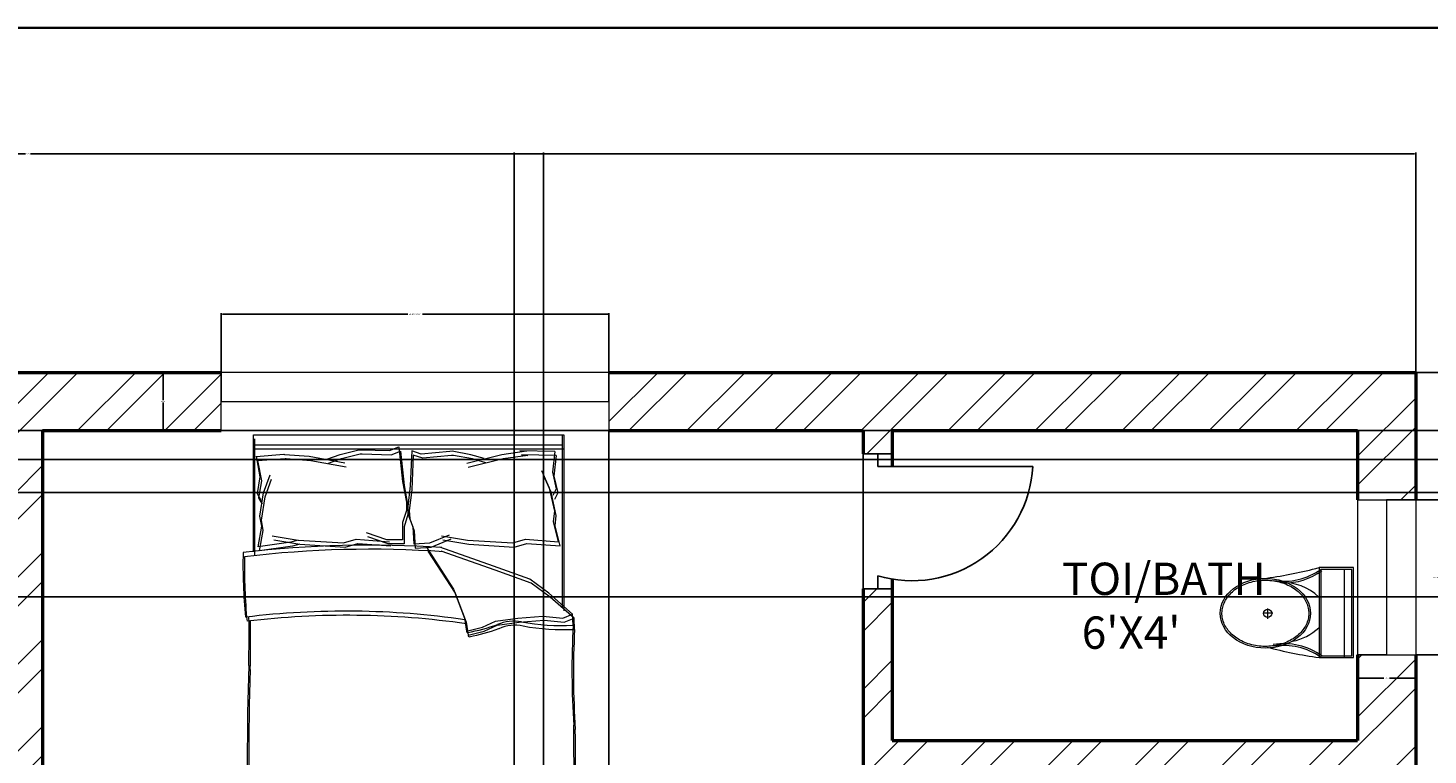
# Model space of a CAD drawing. Units: inches. Extents: x 2310 to 2937, y 1113 to 2410.
# Tile 22 of 23: x 2609 to 2826, y 2297 to 2410. Entities that reach past the tile are written whole.
import ezdxf

# ---------------------------------------------------------------- set-up
doc = ezdxf.new("R2010")
doc.units = ezdxf.units.IN
for name, color, linetype, lineweight in [('A-ANNO-DIMS', 2, 'Continuous', 18), ('A-ANNO-TTLB', 7, 'Continuous', 35), ('A-AREA-IDEN', 7, 'Continuous', 18), ('A-DOOR', 31, 'Continuous', 25), ('A-FLOR-FIXT', 9, 'Continuous', 18), ('A-FURN', 8, 'Continuous', 18), ('A-GLAZ', 191, 'Continuous', 20), ('A-WALL', 7, 'Continuous', 50), ('A-WALL-PATT', 85, 'Continuous', 13)]:
    doc.layers.add(name, color=color, linetype=linetype, lineweight=lineweight)
doc.styles.get("Standard").update_dxf_attribs({"font": 'arial.ttf'})
doc.dimstyles.get("Standard").update_dxf_attribs({"dimtxt": 0.18, "dimasz": 0.18, "dimexe": 0.18, "dimexo": 0.0625, "dimgap": 0.09, "dimtad": 0, "dimtih": 1, "dimtoh": 1, "dimdec": 4, "dimzin": 0, "dimdsep": 46, "dimtxsty": 'Standard', "dimcen": 0.09, "dimadec": 0, "dimazin": 0, "dimtfac": 1, "dimtdec": 4, "dimtofl": 0, "dimtmove": 0, "dimatfit": 3, "dimfxl": 1, "dimtolj": 1, "dimtzin": 0, "dimarcsym": 0})

# ---------------------------------------------------------------- blocks, each defined once
blk = doc.blocks.new('A$C31115884')
for p, q in [((283.1, 497.7), (223.4, 497.7)), ((257.5, 466.4), (257.5, 523.2)), ((0, 200), (0, 0)), ((520, 200), (0, 200)), ((10, 190), (10, 10)), ((510, 190), (10, 190)), ((510, 10), (510, 190)), ((520, 0), (520, 200)), ((510, 54.5), (0, 54.5)), ((10, 10), (510, 10)), ((0, 0), (520, 0))]:
    blk.add_line(p, q)
blk.add_circle((255.6, 496.4), 23.6)
for centre, radius, start, end in [((2777.7, -204.6), 2807, 165.4549, 171.71327), ((3237, 905), 2807, 188.28673, 194.5451), ((-294.5, 403.3), 364.7, 324.20913, 9.34987), ((-294.5, 403.3), 374.7, 324.20913, 9.34987), ((139.5, 406.2), 293.5, 315.84364, 2.65635), ((805.8, 403.3), 374.7, 179.20365, 215.79087), ((805.8, 403.3), 364.7, 170.65013, 215.79087), ((383.6, 406.2), 293.5, 190.27735, 224.15636)]:
    blk.add_arc(centre, radius, start, end)
blk.add_ellipse((256.2, 509.9), major_axis=(0, -260.7), ratio=0.772727)
blk.add_open_spline([(256.2, 259.2), (263.1, 259.2), (270, 259.7), (287.8, 262.3), (298.7, 265.1), (319.9, 273.1), (330.2, 278.4), (350.1, 291.1), (359.7, 298.7), (377.7, 315.9), (386.2, 325.5), (401.7, 346.6), (408.8, 358.1), (421.3, 382.5), (426.8, 395.5), (435.9, 422.4), (439.5, 436.4), (444.8, 465.1), (446.5, 479.7), (447.9, 509.2), (447.6, 524), (445, 553.3), (442.7, 567.8), (436.3, 596), (432.1, 609.7), (421.9, 636), (416, 648.6), (402.5, 672.1), (395, 683), (378.6, 703), (369.8, 712.1), (351.1, 728), (341.3, 734.8), (320.9, 746.2), (310.4, 750.7), (288.9, 757.3), (278, 759.4), (256, 761), (245, 760.6), (223.1, 757.2), (212.3, 754.3), (191.1, 746.1), (180.8, 740.7), (160.9, 727.8), (151.4, 720.1), (133.5, 702.7), (125.1, 693), (109.6, 671.7), (102.6, 660.2), (90.2, 635.7), (84.9, 622.7), (76, 595.6), (72.4, 581.6), (67.2, 552.9), (65.6, 538.2), (64.4, 508.8), (64.8, 494), (67.5, 464.7), (69.9, 450.2), (76.6, 422), (80.8, 408.3), (91.1, 382.2), (97.2, 369.7), (110.8, 346.3), (118.4, 335.4), (134.8, 315.6), (143.7, 306.7), (162.4, 290.9), (172.3, 284.2), (192.8, 273), (203.3, 268.6), (224.8, 262.2), (235.8, 260.2), (249.9, 259.3), (253, 259.2), (256.2, 259.2)], degree=3, knots=[0, 0, 0, 0, 0.110105, 0.110105, 0.285049, 0.285049, 0.459994, 0.459994, 0.634938, 0.634938, 0.809882, 0.809882, 0.984827, 0.984827, 1.159771, 1.159771, 1.334715, 1.334715, 1.50966, 1.50966, 1.684604, 1.684604, 1.859549, 1.859549, 2.034493, 2.034493, 2.209437, 2.209437, 2.384382, 2.384382, 2.559326, 2.559326, 2.73427, 2.73427, 2.909215, 2.909215, 3.084159, 3.084159, 3.259103, 3.259103, 3.434048, 3.434048, 3.608992, 3.608992, 3.783936, 3.783936, 3.958881, 3.958881, 4.133825, 4.133825, 4.30877, 4.30877, 4.483714, 4.483714, 4.658658, 4.658658, 4.833603, 4.833603, 5.008547, 5.008547, 5.183491, 5.183491, 5.358436, 5.358436, 5.53338, 5.53338, 5.708324, 5.708324, 5.883269, 5.883269, 6.058213, 6.058213, 6.233158, 6.233158, 6.283185, 6.283185, 6.283185, 6.283185])
blk = doc.blocks.new('BED-DOUBLE')
for p, q in [((3.56, 63.44), (3.56, 81.55)), ((3.56, 63.44), (3.56, 81.55)), ((3.56, 81.55), (51.58, 81.55)), ((3.79, 62.8), (3.79, 80.91)), ((3.79, 62.8), (3.79, 80.91)), ((51.35, 81.55), (51.35, 54.94)), ((51.35, 81.55), (51.35, 54.94)), ((51.58, 81.55), (51.58, 80.91)), ((51.58, 80.91), (51.58, 54.3)), ((51.58, 80.91), (51.58, 54.3)), ((3.56, 80.01), (51.35, 80.01)), ((3.56, 80.01), (51.35, 80.01)), ((3.79, 79.38), (51.58, 79.38)), ((3.79, 79.38), (51.58, 79.38)), ((3.98, 78.21), (8.27, 78.54)), ((3.98, 78.23), (4.56, 75.05)), ((3.98, 78.23), (4.56, 75.05)), ((3.99, 78.21), (8.27, 78.54)), ((8.27, 78.54), (8.37, 78.52)), ((8.27, 78.54), (8.37, 78.52)), ((8.37, 78.52), (12.19, 78.23)), ((8.37, 78.52), (12.19, 78.23)), ((12.19, 78.23), (17.69, 77.22)), ((12.19, 78.23), (17.69, 77.22)), ((14.94, 77.8), (16.97, 78.52)), ((14.94, 77.8), (16.96, 78.52)), ((16.96, 78.52), (19.86, 79.24)), ((16.97, 78.52), (19.86, 79.24)), ((17.19, 77.88), (20.08, 78.61)), ((17.19, 77.88), (20.08, 78.61)), ((19.86, 79.24), (20.18, 79.24)), ((19.86, 79.24), (20.18, 79.24)), ((20.08, 78.61), (20.41, 78.61)), ((20.08, 78.61), (20.41, 78.61)), ((20.18, 79.24), (24.62, 79.1)), ((20.18, 79.24), (24.62, 79.1)), ((20.41, 78.61), (24.85, 78.46)), ((20.41, 78.61), (24.85, 78.46)), ((24.62, 79.1), (26.07, 79.68)), ((24.62, 79.1), (26.07, 79.68)), ((24.85, 78.46), (26.3, 79.04)), ((24.85, 78.46), (26.3, 79.04)), ((26.07, 79.68), (26.65, 74.33)), ((26.07, 79.68), (26.65, 74.33)), ((26.3, 79.04), (26.88, 73.69)), ((26.3, 79.04), (26.88, 73.69)), ((28.06, 79.06), (27.82, 73.68)), ((28.06, 79.06), (27.82, 73.68)), ((28.29, 78.42), (28.05, 73.04)), ((28.29, 78.42), (28.05, 73.04)), ((29.54, 78.57), (28.06, 79.06)), ((29.54, 78.57), (28.06, 79.06)), ((29.77, 77.93), (28.29, 78.42)), ((29.77, 77.93), (28.29, 78.42)), ((33.97, 78.99), (29.54, 78.57)), ((33.97, 78.99), (29.54, 78.57)), ((34.2, 78.35), (29.77, 77.93)), ((34.2, 78.35), (29.77, 77.93)), ((34.29, 79.01), (33.97, 78.99)), ((34.29, 79.01), (33.97, 78.99)), ((34.52, 78.37), (34.2, 78.35)), ((34.52, 78.37), (34.2, 78.35)), ((37.22, 78.47), (34.29, 79.01)), ((37.22, 78.47), (34.29, 79.01)), ((37.45, 77.83), (34.52, 78.37)), ((37.45, 77.83), (34.52, 78.37)), ((42, 78.48), (36.58, 77.13)), ((42, 78.48), (36.58, 77.13)), ((39.29, 77.87), (37.22, 78.47)), ((39.29, 77.87), (37.22, 78.47)), ((45.8, 79.01), (42, 78.48)), ((45.8, 79.01), (42, 78.48)), ((46.03, 78.37), (42.23, 77.84)), ((46.03, 78.37), (42.23, 77.84)), ((50.2, 78.99), (44.8, 79.09)), ((44.8, 79.09), (45.8, 79.01)), ((50.2, 78.99), (44.8, 79.09)), ((44.8, 79.09), (45.8, 79.01)), ((50.43, 78.35), (45.02, 78.45)), ((45.02, 78.45), (46.03, 78.37)), ((50.43, 78.35), (45.02, 78.45)), ((45.02, 78.45), (46.03, 78.37)), ((50.2, 78.99), (49.82, 75.78)), ((50.2, 78.99), (49.82, 75.78)), ((50.43, 78.35), (50.05, 75.14)), ((50.43, 78.35), (50.05, 75.14)), ((4.21, 77.57), (8.49, 77.9)), ((4.21, 77.57), (8.49, 77.9)), ((4.21, 77.59), (4.79, 74.41)), ((4.21, 77.59), (4.79, 74.41)), ((8.49, 77.9), (8.6, 77.88)), ((8.49, 77.9), (8.6, 77.88)), ((8.6, 77.88), (12.42, 77.59)), ((8.6, 77.88), (12.42, 77.59)), ((12.42, 77.59), (17.92, 76.58)), ((12.42, 77.59), (17.92, 76.58)), ((15.17, 77.16), (17.19, 77.88)), ((15.17, 77.16), (17.19, 77.88)), ((42.23, 77.84), (36.81, 76.49)), ((42.23, 77.84), (36.81, 76.49)), ((39.52, 77.24), (37.45, 77.83)), ((39.51, 77.24), (37.45, 77.83)), ((49.4, 73.29), (48.21, 75.97)), ((49.4, 73.29), (48.21, 75.97)), ((4.56, 75.05), (4.13, 72.45)), ((4.56, 75.05), (4.13, 72.45)), ((4.79, 74.41), (4.35, 71.81)), ((4.79, 74.41), (4.35, 71.81)), ((5.14, 72.59), (6.15, 75.34)), ((5.14, 72.59), (6.15, 75.34)), ((5.37, 71.95), (6.38, 74.7)), ((5.37, 71.95), (6.38, 74.7)), ((26.65, 74.33), (27.23, 71.15)), ((26.65, 74.33), (27.23, 71.15)), ((26.88, 73.69), (27.45, 70.51)), ((26.88, 73.69), (27.45, 70.51)), ((27.82, 73.68), (27.44, 70.47)), ((27.82, 73.68), (27.44, 70.47)), ((49.62, 72.65), (48.44, 75.33)), ((49.62, 72.65), (48.44, 75.33)), ((49.82, 75.78), (50.42, 73.21)), ((49.82, 75.78), (50.41, 73.21)), ((50.05, 75.14), (50.64, 72.57)), ((50.05, 75.14), (50.64, 72.57)), ((4.13, 72.45), (4.7, 71.44)), ((4.13, 72.45), (4.7, 71.44)), ((4.35, 71.81), (4.93, 70.8)), ((4.35, 71.81), (4.93, 70.8)), ((4.56, 68.98), (5.14, 72.59)), ((4.56, 68.98), (5.14, 72.59)), ((4.79, 68.34), (5.37, 71.95)), ((4.79, 68.34), (5.37, 71.95)), ((28.05, 73.04), (27.67, 69.83)), ((28.05, 73.04), (27.67, 69.83)), ((50.2, 69.72), (49.4, 73.29)), ((50.2, 69.72), (49.4, 73.29)), ((50.43, 69.08), (49.62, 72.65)), ((50.43, 69.08), (49.62, 72.65)), ((50.42, 73.21), (49.9, 72.16)), ((50.41, 73.21), (49.9, 72.16)), ((50.64, 72.57), (50.13, 71.52)), ((50.64, 72.57), (50.13, 71.52)), ((27.23, 69.85), (26.65, 67.97)), ((27.23, 69.85), (26.65, 67.97)), ((27.23, 71.15), (27.23, 69.85)), ((27.23, 71.15), (27.23, 69.85)), ((27.44, 70.47), (27.52, 69.17)), ((27.44, 70.47), (27.52, 69.17)), ((27.45, 70.51), (27.45, 69.21)), ((27.45, 70.51), (27.45, 69.21)), ((27.67, 69.83), (27.75, 68.53)), ((27.67, 69.83), (27.75, 68.53)), ((50.01, 68.11), (50.2, 69.72)), ((50.01, 68.11), (50.2, 69.72)), ((4.27, 64.21), (4.85, 67.39)), ((4.27, 64.21), (4.85, 67.39)), ((4.85, 67.39), (4.56, 68.98)), ((4.85, 67.39), (4.56, 68.98)), ((5.08, 66.75), (4.79, 68.34)), ((5.08, 66.75), (4.79, 68.34)), ((26.65, 67.97), (26.65, 65.29)), ((26.65, 67.97), (26.65, 65.29)), ((27.45, 69.21), (26.88, 67.33)), ((27.45, 69.21), (26.88, 67.33)), ((26.88, 67.33), (26.88, 64.65)), ((26.88, 67.33), (26.88, 64.65)), ((27.52, 69.17), (28.22, 67.33)), ((27.52, 69.17), (28.22, 67.33)), ((27.75, 68.53), (28.45, 66.69)), ((27.75, 68.53), (28.44, 66.69)), ((28.22, 67.33), (28.38, 64.66)), ((28.22, 67.33), (28.38, 64.66)), ((50.78, 64.98), (50.01, 68.11)), ((50.78, 64.98), (50.01, 68.11)), ((50.24, 67.48), (50.43, 69.08)), ((50.24, 67.48), (50.43, 69.08)), ((51.01, 64.34), (50.24, 67.48)), ((51.01, 64.34), (50.24, 67.48)), ((4.5, 63.57), (5.08, 66.75)), ((4.5, 63.57), (5.08, 66.75)), ((6.47, 65.92), (10.5, 65.25)), ((6.47, 65.92), (10.5, 65.25)), ((6.7, 65.28), (10.73, 64.61)), ((6.7, 65.28), (10.73, 64.61)), ((10.5, 65.25), (9.37, 64.93)), ((10.5, 65.25), (9.37, 64.93)), ((10.5, 65.25), (17.51, 64.82)), ((10.5, 65.25), (17.51, 64.82)), ((17.51, 64.82), (19.47, 65.38)), ((17.51, 64.82), (19.47, 65.38)), ((19.47, 65.38), (24.6, 64.98)), ((19.47, 65.38), (24.6, 64.98)), ((24.19, 65.29), (21.04, 66.38)), ((24.19, 65.29), (21.05, 66.38)), ((24.42, 64.65), (21.27, 65.74)), ((24.42, 64.65), (21.27, 65.74)), ((26.65, 65.29), (24.19, 65.29)), ((26.65, 65.29), (24.19, 65.29)), ((28.44, 66.69), (28.61, 64.02)), ((28.45, 66.69), (28.61, 64.02)), ((30.84, 64.81), (33.91, 66.09)), ((30.84, 64.81), (33.91, 66.09)), ((31.06, 64.17), (34.14, 65.45)), ((31.07, 64.17), (34.14, 65.45)), ((32.65, 65.92), (36.68, 65.25)), ((32.65, 65.92), (36.68, 65.25)), ((32.88, 65.28), (36.91, 64.61)), ((32.88, 65.28), (36.91, 64.61)), ((36.68, 65.25), (43.69, 64.82)), ((36.68, 65.25), (43.69, 64.82)), ((43.69, 64.82), (45.65, 65.38)), ((43.69, 64.82), (45.65, 65.38)), ((45.65, 65.38), (50.78, 64.98)), ((45.65, 65.38), (50.78, 64.98)), ((9.37, 64.93), (4.27, 64.21)), ((9.37, 64.93), (4.27, 64.21)), ((9.6, 64.29), (4.5, 63.57)), ((9.6, 64.29), (4.5, 63.57)), ((10.73, 64.61), (9.6, 64.29)), ((10.73, 64.61), (9.6, 64.29)), ((10.73, 64.61), (17.74, 64.18)), ((10.73, 64.61), (17.74, 64.18)), ((17.74, 64.18), (19.7, 64.74)), ((17.74, 64.18), (19.7, 64.74)), ((19.7, 64.74), (24.83, 64.34)), ((19.7, 64.74), (24.83, 64.34)), ((26.88, 64.65), (24.42, 64.65)), ((26.88, 64.65), (24.42, 64.65)), ((28.38, 64.66), (30.84, 64.81)), ((28.38, 64.66), (30.84, 64.81)), ((28.61, 64.02), (31.07, 64.17)), ((28.61, 64.02), (31.06, 64.17)), ((30.35, 64.17), (34.54, 57.67)), ((30.35, 64.17), (34.54, 57.67)), ((30.57, 63.53), (34.76, 57.03)), ((30.57, 63.53), (34.76, 57.03)), ((40.73, 61.23), (32.39, 64.17)), ((40.73, 61.23), (32.39, 64.17)), ((40.96, 60.59), (32.62, 63.53)), ((40.96, 60.59), (32.62, 63.53)), ((36.91, 64.61), (43.92, 64.18)), ((36.91, 64.61), (43.92, 64.18)), ((43.92, 64.18), (45.88, 64.74)), ((43.92, 64.18), (45.88, 64.74)), ((45.88, 64.74), (51.01, 64.34)), ((45.88, 64.74), (51.01, 64.34)), ((46.31, 59.22), (40.73, 61.23)), ((46.31, 59.22), (40.73, 61.23)), ((46.53, 58.58), (40.96, 60.59)), ((46.53, 58.58), (40.96, 60.59)), ((49.25, 57.05), (46.31, 59.22)), ((49.25, 57.05), (46.31, 59.22)), ((49.48, 56.41), (46.53, 58.58)), ((49.48, 56.41), (46.53, 58.58)), ((34.54, 57.67), (36.24, 53.18)), ((34.54, 57.67), (36.24, 53.18)), ((34.76, 57.03), (36.47, 52.54)), ((34.76, 57.03), (36.47, 52.54)), ((52.95, 53.8), (49.25, 57.05)), ((52.95, 53.8), (49.25, 57.05)), ((53.18, 53.16), (49.48, 56.41)), ((53.18, 53.16), (49.48, 56.41)), ((36.24, 53.18), (36.55, 51.17)), ((36.24, 53.18), (36.55, 51.17)), ((36.47, 52.54), (36.78, 50.53)), ((36.47, 52.54), (36.78, 50.53)), ((39.03, 51.79), (41.04, 52.72)), ((39.03, 51.79), (41.04, 52.72)), ((39.26, 51.15), (41.27, 52.08)), ((39.26, 51.15), (41.27, 52.08)), ((41.04, 52.72), (44.45, 53.18)), ((41.04, 52.72), (44.45, 53.18)), ((41.27, 52.08), (44.68, 52.54)), ((41.27, 52.08), (44.68, 52.54)), ((44.45, 53.18), (48.32, 53.49)), ((44.45, 53.18), (48.32, 53.49)), ((44.68, 52.54), (48.55, 52.85)), ((44.68, 52.54), (48.55, 52.85)), ((48.32, 53.49), (51.42, 53.18)), ((48.32, 53.49), (51.42, 53.18)), ((48.55, 52.85), (51.65, 52.54)), ((48.55, 52.85), (51.65, 52.54)), ((51.42, 53.18), (52.95, 53.8)), ((51.42, 53.18), (52.95, 53.8)), ((51.65, 52.54), (53.18, 53.16)), ((51.65, 52.54), (53.18, 53.16)), ((53.03, 52.06), (52.95, 53.8, 3.87)), ((53.03, 52.06), (52.95, 53.8, 3.87)), ((53.26, 51.42), (53.18, 53.16, 3.87)), ((53.26, 51.42), (53.18, 53.16, 3.87)), ((36.55, 51.17), (39.03, 51.79)), ((36.55, 51.17), (39.03, 51.79)), ((36.78, 50.53), (39.26, 51.15)), ((36.78, 50.53), (39.26, 51.15)), ((15.15, 2.3), (39.76, 2.3)), ((15.15, 2.3), (39.76, 2.3)), ((15.38, 1.66), (39.99, 1.66)), ((15.38, 1.66), (39.99, 1.66))]:
    blk.add_line(p, q)
for centre, radius, start, end in [((85.25, 61.45), 83.31, 178.7218, 185.604), ((85.25, 61.45), 83.31, 178.7218, 185.604), ((21.45, -100.5), 164.97, 86.0865, 96.7821), ((21.45, -100.5), 164.97, 86.0865, 96.7821), ((21.67, -101.14), 164.97, 86.0865, 96.7821), ((21.67, -101.14), 164.97, 86.0865, 96.7821), ((85.48, 60.81), 83.31, 178.7218, 185.604), ((85.48, 60.81), 83.31, 178.7218, 185.604), ((17.84, -74.77), 129.02, 81.7845, 96.9006), ((17.84, -74.77), 129.02, 81.7845, 96.9006), ((18.07, -75.41), 129.02, 81.7845, 96.9006), ((18.07, -75.41), 129.02, 81.7845, 96.9006), ((-167.22, 50.37), 170.11, 358.4762, 1.0082), ((-167.22, 50.37), 170.11, 358.4762, 1.0082), ((-166.99, 49.74), 170.11, 358.4762, 1.0082), ((-166.99, 49.74), 170.11, 358.4762, 1.0082), ((31.24, 80.07), 29.65, 280.6617, 289.8806), ((31.24, 80.07), 29.65, 280.6617, 289.8806), ((43.83, 46.48), 6.22, 78.6608, 113.7384), ((43.83, 46.48), 6.22, 78.6608, 113.7384), ((44.06, 45.84), 6.22, 78.6608, 113.7384), ((44.06, 45.84), 6.22, 78.6608, 113.7384), ((51.41, 88.2), 36.18, 259.8763, 272.5657), ((51.41, 88.2), 36.18, 259.8763, 272.5657), ((182.35, 45.23), 129.5, 176.9791, 183.8365), ((182.35, 45.23), 129.5, 176.9791, 183.8365), ((36.72, 51.11), 0.185, 160.2464, 271.1377), ((36.72, 51.11), 0.185, 160.2464, 271.1377), ((36.95, 50.47), 0.185, 160.2464, 271.1377), ((36.95, 50.47), 0.185, 160.2464, 271.1377), ((31.47, 79.43), 29.65, 280.6617, 289.8806), ((31.47, 79.43), 29.65, 280.6617, 289.8806), ((51.64, 87.57), 36.18, 259.8763, 272.5657), ((51.64, 87.57), 36.18, 259.8763, 272.5657), ((182.58, 44.59), 129.5, 176.9791, 183.8365), ((182.58, 44.59), 129.5, 176.9791, 183.8365), ((484.91, 30.93), 482.31, 178.2277, 181.7185), ((484.91, 30.93), 482.31, 178.2277, 181.7185), ((485.14, 30.3), 482.31, 178.2277, 181.7185), ((485.14, 30.3), 482.31, 178.2277, 181.7185), ((-4508.66, 13.73), 4561.86, 0.00217, 0.28689), ((-4508.66, 13.73), 4561.86, 0.00217, 0.28689), ((-4508.43, 13.09), 4561.86, 0.00217, 0.28689), ((-4508.43, 13.09), 4561.86, 0.00217, 0.28689), ((-26.81, 17.03), 29.63, 346.0648, 358.9113), ((-26.81, 17.03), 29.63, 346.0648, 358.9113), ((-26.58, 16.39), 29.63, 346.0648, 358.9113), ((-26.58, 16.39), 29.63, 346.0648, 358.9113), ((76.24, 12.88), 23.07, 177.4714, 206.4681), ((76.24, 12.88), 23.07, 177.4714, 206.4681), ((76.47, 12.24), 23.07, 177.4714, 206.4681), ((76.47, 12.24), 23.07, 177.4714, 206.4681), ((-21.57, 11.27), 23.56, 337.9751, 356.652), ((-21.57, 11.27), 23.56, 337.9751, 356.652), ((-21.34, 10.63), 23.56, 337.9751, 356.652), ((-21.34, 10.63), 23.56, 337.9751, 356.652), ((1.17, 1.83), 1.09, 146.1736, 293.4781), ((1.17, 1.83), 1.09, 146.1736, 293.4781), ((21.51, -119.29), 121.76, 92.9958, 99.4091), ((21.51, -119.29), 121.76, 92.9958, 99.4091), ((-17.14, 105.26), 106.46, 283.3832, 287.7053), ((-17.14, 105.26), 106.46, 283.3832, 287.7053), ((-16.91, 104.62), 106.46, 283.3832, 287.7053), ((-16.91, 104.62), 106.46, 283.3832, 287.7053), ((41.24, -130.73), 133.04, 84.4998, 90.6351), ((41.24, -130.73), 133.04, 84.4998, 90.6351), ((54.5, 2.68), 1.1, 242.6588, 356.02), ((54.5, 2.68), 1.1, 242.6588, 356.02), ((1.4, 1.19), 1.09, 146.1736, 293.4781), ((1.4, 1.19), 1.09, 146.1736, 293.4781), ((21.74, -119.93), 121.76, 92.9958, 99.4091), ((21.74, -119.93), 121.76, 92.9958, 99.4091), ((41.47, -131.37), 133.04, 84.4998, 90.6351), ((41.47, -131.37), 133.04, 84.4998, 90.6351), ((54.72, 2.04), 1.1, 242.6588, 356.02), ((54.72, 2.04), 1.1, 242.6588, 356.02)]:
    blk.add_arc(centre, radius, start, end)
blk = doc.blocks.new('WIN-24IN')
for p, q in [((0, 24), (9, 24)), ((0, 24), (0, 0)), ((9, 24), (4.5, 24)), ((4.5, 24), (4.5, 0)), ((9, 24), (9, 0)), ((4.5, 0), (0, 0)), ((0, 0), (9, 0))]:
    blk.add_line(p, q)
blk = doc.blocks.new('WIN-60IN-HEAD')
for p, q in [((0, 0), (0, 9)), ((0, 9), (0, 4.5)), ((60, 9), (0, 9)), ((60, 4.5), (60, 9)), ((60, 9), (60, 0)), ((0, 4.5), (60, 4.5)), ((0, 0), (60, 0))]:
    blk.add_line(p, q)
blk = doc.blocks.new('*D29')
at = {"layer": 'A-ANNO-DIMS', "color": 0, "lineweight": -2, "transparency": 16777216}
for p, q in [((2824.05, 2336.76), (2827.77, 2336.76)), ((2827.59, 2336.58), (2827.59, 2324.94)), ((2827.59, 2312.94), (2827.59, 2324.58)), ((2824.05, 2312.76), (2827.77, 2312.76))]:
    blk.add_line(p, q, dxfattribs=at)
at = {"layer": 'A-ANNO-DIMS', "color": 0, "transparency": 16777216}
for points in [[(2827.56, 2336.58), (2827.62, 2336.58), (2827.59, 2336.76)], [(2827.56, 2312.94), (2827.62, 2312.94), (2827.59, 2312.76)]]:
    blk.add_solid(points, dxfattribs=at)
at = {"layer": 'Defpoints', "color": 0, "transparency": 16777216}
for p in [(2823.99, 2336.76), (2827.59, 2336.76), (2823.99, 2312.76)]:
    blk.add_point(p, dxfattribs=at)
at = {"layer": 'A-ANNO-DIMS', "color": 0, "transparency": 16777216, "insert": (2827.59, 2324.76), "char_height": 0.18, "attachment_point": 5}
blk.add_mtext('\\A1;WINDOW 24 TYP.', dxfattribs=at)
blk = doc.blocks.new('*D30')
at = {"layer": 'A-ANNO-DIMS', "color": 0, "lineweight": -2, "transparency": 16777216}
for p, q in [((2814.99, 2312.7), (2814.99, 2308.98)), ((2823.99, 2312.7), (2823.99, 2308.98)), ((2815.17, 2309.16), (2819.03, 2309.16)), ((2823.81, 2309.16), (2819.94, 2309.16))]:
    blk.add_line(p, q, dxfattribs=at)
at = {"layer": 'A-ANNO-DIMS', "color": 0, "transparency": 16777216}
for points in [[(2815.17, 2309.19), (2815.17, 2309.13), (2814.99, 2309.16)], [(2823.81, 2309.19), (2823.81, 2309.13), (2823.99, 2309.16)]]:
    blk.add_solid(points, dxfattribs=at)
at = {"layer": 'Defpoints', "color": 0, "transparency": 16777216}
for p in [(2814.99, 2312.76), (2823.99, 2312.76), (2823.99, 2309.16)]:
    blk.add_point(p, dxfattribs=at)
at = {"layer": 'A-ANNO-DIMS', "color": 0, "transparency": 16777216, "insert": (2819.49, 2309.16), "char_height": 0.18, "attachment_point": 5}
blk.add_mtext('\\A1;9 TYP.', dxfattribs=at)
blk = doc.blocks.new('*D33')
at = {"layer": 'A-ANNO-DIMS', "color": 0, "lineweight": -2, "transparency": 16777216}
for p, q in [((2639.14, 2356.58), (2639.14, 2365.69)), ((2639.32, 2365.51), (2668.02, 2365.51)), ((2698.96, 2365.51), (2670.26, 2365.51)), ((2699.14, 2356.58), (2699.14, 2365.69))]:
    blk.add_line(p, q, dxfattribs=at)
at = {"layer": 'A-ANNO-DIMS', "color": 0, "transparency": 16777216}
for points in [[(2639.32, 2365.54), (2639.32, 2365.48), (2639.14, 2365.51)], [(2698.96, 2365.54), (2698.96, 2365.48), (2699.14, 2365.51)]]:
    blk.add_solid(points, dxfattribs=at)
at = {"layer": 'Defpoints', "color": 0, "transparency": 16777216}
for p in [(2699.14, 2365.51), (2639.14, 2356.51), (2699.14, 2356.51)]:
    blk.add_point(p, dxfattribs=at)
at = {"layer": 'A-ANNO-DIMS', "color": 0, "transparency": 16777216, "insert": (2669.14, 2365.51), "char_height": 0.18, "attachment_point": 5}
blk.add_mtext('\\A1;WINDOW 60 TYP.', dxfattribs=at)
blk = doc.blocks.new('*D34')
at = {"layer": 'A-ANNO-DIMS', "color": 0, "lineweight": -2, "transparency": 16777216}
for p, q in [((2639.08, 2356.51), (2629.96, 2356.51)), ((2630.14, 2356.33), (2630.14, 2352.2)), ((2630.14, 2347.69), (2630.14, 2351.83)), ((2639.08, 2347.51), (2629.96, 2347.51))]:
    blk.add_line(p, q, dxfattribs=at)
at = {"layer": 'A-ANNO-DIMS', "color": 0, "transparency": 16777216}
for points in [[(2630.11, 2356.33), (2630.17, 2356.33), (2630.14, 2356.51)], [(2630.11, 2347.69), (2630.17, 2347.69), (2630.14, 2347.51)]]:
    blk.add_solid(points, dxfattribs=at)
at = {"layer": 'Defpoints', "color": 0, "transparency": 16777216}
for p in [(2630.14, 2356.51), (2639.14, 2356.51), (2639.14, 2347.51)]:
    blk.add_point(p, dxfattribs=at)
at = {"layer": 'A-ANNO-DIMS', "color": 0, "transparency": 16777216, "insert": (2630.14, 2352.01), "char_height": 0.18, "attachment_point": 5}
blk.add_mtext('\\A1;9 TYP.', dxfattribs=at)
blk = doc.blocks.new('*D39')
at = {"layer": 'A-ANNO-DIMS', "color": 0, "lineweight": -2, "transparency": 16777216}
for p, q in [((2394.49, 2356.58), (2394.49, 2390.54)), ((2394.67, 2390.36), (2608.84, 2390.36)), ((2823.81, 2390.36), (2609.63, 2390.36)), ((2823.99, 2356.58), (2823.99, 2390.54))]:
    blk.add_line(p, q, dxfattribs=at)
at = {"layer": 'A-ANNO-DIMS', "color": 0, "transparency": 16777216}
for points in [[(2394.67, 2390.39), (2394.67, 2390.33), (2394.49, 2390.36)], [(2823.81, 2390.39), (2823.81, 2390.33), (2823.99, 2390.36)]]:
    blk.add_solid(points, dxfattribs=at)
at = {"layer": 'Defpoints', "color": 0, "transparency": 16777216}
for p in [(2823.99, 2390.36), (2394.49, 2356.51), (2823.99, 2356.51)]:
    blk.add_point(p, dxfattribs=at)
at = {"layer": 'A-ANNO-DIMS', "color": 0, "transparency": 16777216, "insert": (2609.24, 2390.36), "char_height": 0.18, "attachment_point": 5}
blk.add_mtext('\\A1;429.5', dxfattribs=at)
blk = doc.blocks.new('*D42')
at = {"layer": 'A-ANNO-DIMS', "color": 0, "lineweight": -2, "transparency": 16777216}
for p, q in [((2699.14, 2347.45), (2699.14, 1649.5)), ((2738.49, 2347.45), (2738.49, 1649.5)), ((2699.32, 1649.68), (2718.42, 1649.68)), ((2738.31, 1649.68), (2719.21, 1649.68))]:
    blk.add_line(p, q, dxfattribs=at)
at = {"layer": 'A-ANNO-DIMS', "color": 0, "transparency": 16777216}
for points in [[(2699.32, 1649.71), (2699.32, 1649.65), (2699.14, 1649.68)], [(2738.31, 1649.71), (2738.31, 1649.65), (2738.49, 1649.68)]]:
    blk.add_solid(points, dxfattribs=at)
at = {"layer": 'Defpoints', "color": 0, "transparency": 16777216}
for p in [(2699.14, 2347.51), (2738.49, 2347.51), (2738.49, 1649.68)]:
    blk.add_point(p, dxfattribs=at)
at = {"layer": 'A-ANNO-DIMS', "color": 0, "transparency": 16777216, "insert": (2718.81, 1649.68), "char_height": 0.18, "attachment_point": 5}
blk.add_mtext('\\A1;39.35', dxfattribs=at)
blk = doc.blocks.new('*D50')
at = {"layer": 'A-ANNO-DIMS', "color": 0, "lineweight": -2, "transparency": 16777216}
for p, q in [((2824.05, 2312.76), (2858.02, 2312.76)), ((2857.84, 2312.58), (2857.84, 2291.51)), ((2857.84, 2270.08), (2857.84, 2291.15)), ((2824.05, 2269.9), (2858.02, 2269.9))]:
    blk.add_line(p, q, dxfattribs=at)
at = {"layer": 'A-ANNO-DIMS', "color": 0, "transparency": 16777216}
for points in [[(2857.81, 2312.58), (2857.87, 2312.58), (2857.84, 2312.76)], [(2857.81, 2270.08), (2857.87, 2270.08), (2857.84, 2269.9)]]:
    blk.add_solid(points, dxfattribs=at)
at = {"layer": 'Defpoints', "color": 0, "transparency": 16777216}
for p in [(2823.99, 2312.76), (2857.84, 2312.76), (2823.99, 2269.9)]:
    blk.add_point(p, dxfattribs=at)
at = {"layer": 'A-ANNO-DIMS', "color": 0, "transparency": 16777216, "insert": (2857.84, 2291.33), "char_height": 0.18, "attachment_point": 5}
blk.add_mtext('\\A1;42.86', dxfattribs=at)
blk = doc.blocks.new('*D51')
at = {"layer": 'A-ANNO-DIMS', "color": 0, "lineweight": -2, "transparency": 16777216}
for p, q in [((2824.05, 2356.51), (2858.02, 2356.51)), ((2857.84, 2356.33), (2857.84, 2346.82)), ((2857.84, 2336.94), (2857.84, 2346.46)), ((2824.05, 2336.76), (2858.02, 2336.76))]:
    blk.add_line(p, q, dxfattribs=at)
at = {"layer": 'A-ANNO-DIMS', "color": 0, "transparency": 16777216}
for points in [[(2857.81, 2356.33), (2857.87, 2356.33), (2857.84, 2356.51)], [(2857.81, 2336.94), (2857.87, 2336.94), (2857.84, 2336.76)]]:
    blk.add_solid(points, dxfattribs=at)
at = {"layer": 'Defpoints', "color": 0, "transparency": 16777216}
for p in [(2823.99, 2356.51), (2857.84, 2356.51), (2823.99, 2336.76)]:
    blk.add_point(p, dxfattribs=at)
at = {"layer": 'A-ANNO-DIMS', "color": 0, "transparency": 16777216, "insert": (2857.84, 2346.64), "char_height": 0.18, "attachment_point": 5}
blk.add_mtext('\\A1;19.754', dxfattribs=at)
blk = doc.blocks.new('*D52')
at = {"layer": 'A-ANNO-DIMS', "color": 0, "lineweight": -2, "transparency": 16777216}
for p, q in [((2403.55, 2347.51), (2858.02, 2347.51)), ((2857.84, 2347.33), (2857.84, 2342.9)), ((2857.84, 2338.1), (2857.84, 2342.54)), ((2403.55, 2337.92), (2858.02, 2337.92))]:
    blk.add_line(p, q, dxfattribs=at)
at = {"layer": 'A-ANNO-DIMS', "color": 0, "transparency": 16777216}
for points in [[(2857.81, 2347.33), (2857.87, 2347.33), (2857.84, 2347.51)], [(2857.81, 2338.1), (2857.87, 2338.1), (2857.84, 2337.92)]]:
    blk.add_solid(points, dxfattribs=at)
at = {"layer": 'Defpoints', "color": 0, "transparency": 16777216}
for p in [(2403.49, 2347.51), (2403.49, 2337.92), (2857.84, 2337.92)]:
    blk.add_point(p, dxfattribs=at)
at = {"layer": 'A-ANNO-DIMS', "color": 0, "transparency": 16777216, "insert": (2857.84, 2342.72), "char_height": 0.18, "attachment_point": 5}
blk.add_mtext('\\A1;9.59', dxfattribs=at)
blk = doc.blocks.new('*D59')
at = {"layer": 'A-ANNO-DIMS', "color": 0, "lineweight": -2, "transparency": 16777216}
for p, q in [((2480.05, 2343.04), (2858.02, 2343.04)), ((2857.84, 2342.86), (2857.84, 2332.58)), ((2857.84, 2321.94), (2857.84, 2332.22)), ((2480.05, 2321.76), (2858.02, 2321.76))]:
    blk.add_line(p, q, dxfattribs=at)
at = {"layer": 'A-ANNO-DIMS', "color": 0, "transparency": 16777216}
for points in [[(2857.81, 2342.86), (2857.87, 2342.86), (2857.84, 2343.04)], [(2857.81, 2321.94), (2857.87, 2321.94), (2857.84, 2321.76)]]:
    blk.add_solid(points, dxfattribs=at)
at = {"layer": 'Defpoints', "color": 0, "transparency": 16777216}
for p in [(2479.99, 2343.04), (2857.84, 2343.04), (2479.99, 2321.76)]:
    blk.add_point(p, dxfattribs=at)
at = {"layer": 'A-ANNO-DIMS', "color": 0, "transparency": 16777216, "insert": (2857.84, 2332.4), "char_height": 0.18, "attachment_point": 5}
blk.add_mtext('\\A1;21.28', dxfattribs=at)
blk = doc.blocks.new('*D68')
at = {"layer": 'A-ANNO-DIMS', "color": 0, "lineweight": -2, "transparency": 16777216}
for p, q in [((2684.49, 1999.58), (2684.49, 2390.54)), ((2684.67, 2390.36), (2686.48, 2390.36)), ((2688.81, 2390.36), (2686.99, 2390.36)), ((2688.99, 1999.58), (2688.99, 2390.54))]:
    blk.add_line(p, q, dxfattribs=at)
at = {"layer": 'A-ANNO-DIMS', "color": 0, "transparency": 16777216}
for points in [[(2684.67, 2390.39), (2684.67, 2390.33), (2684.49, 2390.36)], [(2688.81, 2390.39), (2688.81, 2390.33), (2688.99, 2390.36)]]:
    blk.add_solid(points, dxfattribs=at)
at = {"layer": 'Defpoints', "color": 0, "transparency": 16777216}
for p in [(2688.99, 2390.36), (2684.49, 1999.51), (2688.99, 1999.51)]:
    blk.add_point(p, dxfattribs=at)
at = {"layer": 'A-ANNO-DIMS', "color": 0, "transparency": 16777216, "insert": (2686.74, 2390.36), "char_height": 0.18, "attachment_point": 5}
blk.add_mtext('\\A1;4.5', dxfattribs=at)

msp = doc.modelspace()

# ---------------------------------------------------------------- hatches: boundary and pattern name
at = {"layer": 'A-WALL-PATT'}
h = msp.add_hatch(dxfattribs=at)
h.set_pattern_fill('ANSI32', color=256)
h.paths.add_polyline_path([(2639.1394, 2356.5139), (2563.662, 2356.5139), (2563.662, 2347.5139), (2606.9859, 2347.5139), (2606.9859, 2210.5139), (2514.2692, 2210.5139), (2514.2692, 2206.0139), (2606.9859, 2206.0139), (2606.9859, 2098.0139), (2602.689, 2098.0139), (2602.689, 2093.5139), (2615.5262, 2093.5139), (2615.5262, 2095.7639), (2615.5262, 2098.0139), (2611.4859, 2098.0139), (2611.4859, 2206.0139), (2703.9391, 2206.0139), (2703.9391, 2208.2639), (2703.9391, 2210.5139), (2611.4859, 2210.5139), (2611.4859, 2347.5139), (2639.1394, 2347.5139)])
h.paths.add_polyline_path([(2823.9859, 2356.5139), (2699.1394, 2356.5139), (2699.1394, 2347.5139), (2738.4859, 2347.5139), (2738.4859, 2343.9266), (2742.9859, 2343.9266), (2742.9859, 2347.5139), (2814.9859, 2347.5139), (2814.9859, 2336.76), (2823.9859, 2336.76)])
h.paths.add_polyline_path([(2823.9859, 2312.76), (2814.9859, 2312.76), (2814.9859, 2299.5139), (2742.9859, 2299.5139), (2742.9859, 2323.0159), (2740.7359, 2323.0159), (2738.4859, 2323.0159), (2738.4859, 2210.5139), (2734.5483, 2210.5139), (2734.5483, 2206.0139), (2746.8769, 2206.0139), (2746.8769, 2208.2639), (2746.8769, 2210.5139), (2742.9859, 2210.5139), (2742.9859, 2295.0139), (2814.9859, 2295.0139), (2814.9859, 2269.8977), (2823.9859, 2269.8977)])
h.paths.add_polyline_path([(2823.9859, 2210.5139), (2823.9859, 2233.8977), (2819.4859, 2233.8977), (2814.9859, 2233.8977), (2814.9859, 2210.5139), (2769.9745, 2210.5139), (2769.9745, 2206.0139), (2814.9859, 2206.0139), (2814.9859, 2178.3027), (2823.9859, 2178.3027)])
h.paths.add_polyline_path([(2823.9859, 2118.3027), (2819.4859, 2118.3027), (2814.9859, 2118.3027), (2814.9859, 2098.0139), (2647.0333, 2098.0139), (2647.0333, 2093.5139), (2814.9859, 2093.5139), (2814.9859, 1999.5139), (2650.6052, 1999.5139), (2650.6052, 1995.0139), (2814.9859, 1995.0139), (2814.9859, 1969.9784), (2823.9859, 1969.9784)])
h.paths.add_polyline_path([(2403.4859, 2093.5139), (2569.9888, 2093.5139), (2569.9888, 2095.7639), (2569.9888, 2098.0139), (2403.4859, 2098.0139), (2403.4859, 2131.7587), (2394.4859, 2131.7587), (2394.4859, 1967.522), (2403.4859, 1967.522), (2403.4859, 1995.0139), (2569.8903, 1995.0139), (2569.8903, 1997.2639), (2569.8903, 1999.5139), (2403.4859, 1999.5139)])
h.paths.add_polyline_path([(2503.662, 2356.5139), (2394.4859, 2356.5139), (2394.4859, 2337.9231), (2398.9859, 2337.9231), (2403.4859, 2337.9231), (2403.4859, 2347.5139), (2475.4859, 2347.5139), (2475.4859, 2343.0384), (2479.9859, 2343.0384), (2479.9859, 2347.5139), (2503.662, 2347.5139)])
h.paths.add_polyline_path([(2498.3065, 1745.5139), (2479.9859, 1745.5139), (2479.9859, 1749.1663), (2477.7359, 1749.1663), (2475.4859, 1749.1663), (2475.4859, 1745.5139), (2403.4859, 1745.5139), (2403.4859, 1753.6409), (2398.9859, 1753.6409), (2394.4859, 1753.6409), (2394.4859, 1736.5139), (2498.3065, 1736.5139), (2498.3065, 1741.0139)])
h.paths.add_polyline_path([(2479.9859, 1882.5139), (2483.9367, 1882.5139), (2483.9367, 1887.0139), (2471.5501, 1887.0139), (2471.5501, 1885.1969), (2471.5501, 1882.5139), (2475.4859, 1882.5139), (2475.4859, 1798.0139), (2403.4859, 1798.0139), (2403.4859, 1828.0433), (2402.2852, 1828.0433), (2394.4859, 1828.0433), (2394.4859, 1777.6409), (2403.4859, 1777.6409), (2403.4859, 1793.5139), (2475.4859, 1793.5139), (2475.4859, 1769.1696), (2479.9859, 1769.1696)])
h.paths.add_polyline_path([(2403.4859, 1907.522), (2398.9859, 1907.522), (2394.4859, 1907.522), (2394.4859, 1864.0433), (2403.4859, 1864.0433), (2403.4859, 1882.5139), (2448.9325, 1882.5139), (2448.9325, 1884.7639), (2448.9325, 1887.0139), (2403.4859, 1887.0139)])
h.paths.add_polyline_path([(2702.2061, 1887.0139), (2611.4859, 1887.0139), (2611.4859, 1995.0139), (2615.6132, 1995.0139), (2615.6132, 1999.5139), (2602.4798, 1999.5139), (2602.4798, 1997.2639), (2602.4798, 1995.0139), (2606.9859, 1995.0139), (2606.9859, 1887.0139), (2516.2443, 1887.0139), (2516.2443, 1884.7639), (2516.2443, 1882.5139), (2606.9859, 1882.5139), (2606.9859, 1745.5139), (2558.3065, 1745.5139), (2558.3065, 1736.5139), (2638.8921, 1736.5139), (2638.8921, 1741.0139), (2638.8921, 1745.5139), (2611.4859, 1745.5139), (2611.4859, 1882.5139), (2702.2061, 1882.5139)])
h.paths.add_polyline_path([(2823.9859, 1909.9784), (2819.4859, 1909.9784), (2814.9859, 1909.9784), (2814.9859, 1887.0139), (2769.144, 1887.0139), (2769.144, 1884.7639), (2769.144, 1882.5139), (2814.9859, 1882.5139), (2814.9859, 1854.1704), (2823.9859, 1854.1704)])
h.paths.add_polyline_path([(2823.9859, 1818.1704), (2819.4859, 1818.1704), (2814.9859, 1818.1704), (2814.9859, 1798.0139), (2742.9859, 1798.0139), (2742.9859, 1882.5139), (2746.805, 1882.5139), (2746.805, 1887.0139), (2733.7334, 1887.0139), (2733.7334, 1884.7639), (2733.7334, 1882.5139), (2738.4859, 1882.5139), (2738.4859, 1771.1728), (2740.7359, 1771.1728), (2742.9859, 1771.1728), (2742.9859, 1793.5139), (2814.9859, 1793.5139), (2814.9859, 1783.6684), (2823.9859, 1783.6684)])
h.paths.add_polyline_path([(2823.9859, 1759.6684), (2814.9859, 1759.6684), (2814.9859, 1745.5139), (2742.9859, 1745.5139), (2742.9859, 1748.9831), (2740.7359, 1748.9831), (2738.4859, 1748.9831), (2738.4859, 1745.5139), (2698.8921, 1745.5139), (2698.8921, 1736.5139), (2823.9859, 1736.5139)])

# ---------------------------------------------------------------- linework, layer by layer
at = {"layer": 'A-ANNO-TTLB'}
msp.add_lwpolyline([(2310.2498, 2409.8427), (2937.0534, 2409.8427), (2937.0534, 1616.036), (2310.2498, 1616.036)], close=True, dxfattribs=at)
at = {"layer": 'A-DOOR'}
for p, q in [((2738.4859, 2343.9266), (2742.9859, 2343.9266)), ((2742.9859, 2343.9266), (2740.7359, 2343.9266)), ((2740.7359, 2343.9266), (2740.7359, 2341.9266)), ((2740.7359, 2341.9266), (2764.7359, 2341.9266)), ((2740.7359, 2323.0159), (2740.7359, 2325.0159)), ((2738.4859, 2323.0159), (2742.9859, 2323.0159)), ((2742.9859, 2323.0159), (2740.7359, 2323.0159))]:
    msp.add_line(p, q, dxfattribs=at)
msp.add_arc((2746.0376, 2342.9777), 18.7279, 253.555369, 356.782643, dxfattribs=at)
at = {"layer": 'A-WALL'}
for p, q in [((2563.662, 2356.5139), (2639.1394, 2356.5139)), ((2699.1394, 2356.5139), (2823.9859, 2356.5139)), ((2823.9859, 2356.5139), (2823.9859, 2336.76)), ((2611.4859, 2347.5139), (2611.4859, 2210.5139)), ((2611.4859, 2347.5139), (2639.1394, 2347.5139)), ((2699.1394, 2347.5139), (2738.4859, 2347.5139)), ((2738.4859, 2347.5139), (2738.4859, 2343.9266)), ((2742.9859, 2347.5139), (2742.9859, 2341.9266)), ((2742.9859, 2347.5139), (2814.9859, 2347.5139)), ((2814.9859, 2347.5139), (2814.9859, 2336.76)), ((2738.4859, 2323.0159), (2738.4859, 2210.5139)), ((2742.9859, 2324.5001), (2742.9859, 2299.5139)), ((2814.9859, 2312.76), (2814.9859, 2299.5139)), ((2823.9859, 2312.76), (2823.9859, 2269.8977)), ((2742.9859, 2299.5139), (2814.9859, 2299.5139))]:
    msp.add_line(p, q, dxfattribs=at)

# ---------------------------------------------------------------- block references
at = {"layer": 'A-FLOR-FIXT', "xscale": 0.0268011493576733, "yscale": 0.0268011493576733, "zscale": 0.0268011493576733, "rotation": 89.99999999999999}
msp.add_blockref('A$C31115884', (2814.3801, 2312.3447), dxfattribs=at)
at = {"layer": 'A-FURN'}
msp.add_blockref('BED-DOUBLE', (2640.5618, 2265.2919), dxfattribs=at)
at = {"layer": 'A-GLAZ'}
for name, p in [('WIN-60IN-HEAD', (2639.1394, 2347.5139)), ('WIN-24IN', (2814.9859, 2312.76))]:
    msp.add_blockref(name, p, dxfattribs=at)

# ---------------------------------------------------------------- texts
at = {"layer": 'A-AREA-IDEN', "insert": (2763.1392, 2327.0496), "char_height": 5, "attachment_point": 1}
msp.add_mtext_dynamic_manual_height_columns("    TOI/BATH\\P      6'X4'", width=82.634083, gutter_width=12.5, heights=[0], dxfattribs=at)

# ---------------------------------------------------------------- dimensions: what is measured, and where the dimension line sits
at = {"layer": 'A-ANNO-DIMS'}
for base, p1, p2, override, picture, middle in [((2823.9859, 2390.3639), (2394.4859, 2356.5139), (2823.9859, 2356.5139), {"dimdec": 1, "dimlfac": 1, "dimrnd": 0, "dimzin": 0, "dimdsep": 46, "dimlunit": 2}, '*D39', (2609.2359, 2390.3639)), ((2688.9859, 2390.3639), (2684.4859, 1999.5139), (2688.9859, 1999.5139), {"dimdec": 1, "dimlfac": 1, "dimrnd": 0, "dimzin": 0, "dimdsep": 46, "dimlunit": 2}, '*D68', (2686.7359, 2390.3639)), ((2738.4859, 1649.6807), (2699.1394, 2347.5139), (2738.4859, 2347.5139), {"dimdec": 2, "dimlfac": 1, "dimrnd": 0, "dimzin": 0, "dimdsep": 46, "dimlunit": 2}, '*D42', (2718.8127, 1649.6807))]:
    dim = msp.add_linear_dim(base=base, p1=p1, p2=p2, dimstyle='Standard', override=override, dxfattribs=at)
    dim.commit()
    dim.dimension.update_dxf_attribs({"geometry": picture, "text_midpoint": middle})
for base, p1, p2, text, picture, middle in [((2699.1394, 2365.5139), (2639.1394, 2356.5139), (2699.1394, 2356.5139), 'WINDOW <> TYP.', '*D33', (2669.1394, 2365.5139)), ((2823.9859, 2309.16), (2814.9859, 2312.76), (2823.9859, 2312.76), '<> TYP.', '*D30', (2819.4859, 2309.16))]:
    dim = msp.add_linear_dim(base=base, p1=p1, p2=p2, text=text, dimstyle='Standard', override={"dimdec": 0, "dimlfac": 1, "dimrnd": 0, "dimzin": 0, "dimdsep": 46, "dimlunit": 2}, dxfattribs=at)
    dim.commit()
    dim.dimension.update_dxf_attribs({"geometry": picture, "text_midpoint": middle})
for base, p1, p2, text, picture, middle in [((2630.1394, 2356.5139), (2639.1394, 2347.5139), (2639.1394, 2356.5139), '<> TYP.', '*D34', (2630.1394, 2352.0139)), ((2827.5859, 2336.76), (2823.9859, 2312.76), (2823.9859, 2336.76), 'WINDOW <> TYP.', '*D29', (2827.5859, 2324.76))]:
    dim = msp.add_linear_dim(base=base, p1=p1, p2=p2, angle=90, text=text, dimstyle='Standard', override={"dimdec": 0, "dimlfac": 1, "dimrnd": 0, "dimzin": 0, "dimdsep": 46, "dimlunit": 2}, dxfattribs=at)
    dim.commit()
    dim.dimension.update_dxf_attribs({"geometry": picture, "text_midpoint": middle})
for base, p1, p2, override, picture, middle in [((2857.8359, 2356.5139), (2823.9859, 2336.76), (2823.9859, 2356.5139), {"dimdec": 3, "dimlfac": 1, "dimrnd": 0, "dimzin": 0, "dimdsep": 46, "dimlunit": 2}, '*D51', (2857.8359, 2346.637)), ((2857.8359, 2337.9231), (2403.4859, 2347.5139), (2403.4859, 2337.9231), {"dimdec": 2, "dimlfac": 1, "dimrnd": 0, "dimzin": 0, "dimdsep": 46, "dimlunit": 2}, '*D52', (2857.8359, 2342.7185)), ((2857.8359, 2343.0384), (2479.9859, 2321.7598), (2479.9859, 2343.0384), {"dimdec": 2, "dimlfac": 1, "dimrnd": 0, "dimzin": 0, "dimdsep": 46, "dimlunit": 2}, '*D59', (2857.8359, 2332.3991)), ((2857.8359, 2312.76), (2823.9859, 2269.8977), (2823.9859, 2312.76), {"dimdec": 2, "dimlfac": 1, "dimrnd": 0, "dimzin": 0, "dimdsep": 46, "dimlunit": 2}, '*D50', (2857.8359, 2291.3288))]:
    dim = msp.add_linear_dim(base=base, p1=p1, p2=p2, angle=90, dimstyle='Standard', override=override, dxfattribs=at)
    dim.commit()
    dim.dimension.update_dxf_attribs({"geometry": picture, "text_midpoint": middle})

doc.saveas('drawing.dxf')
